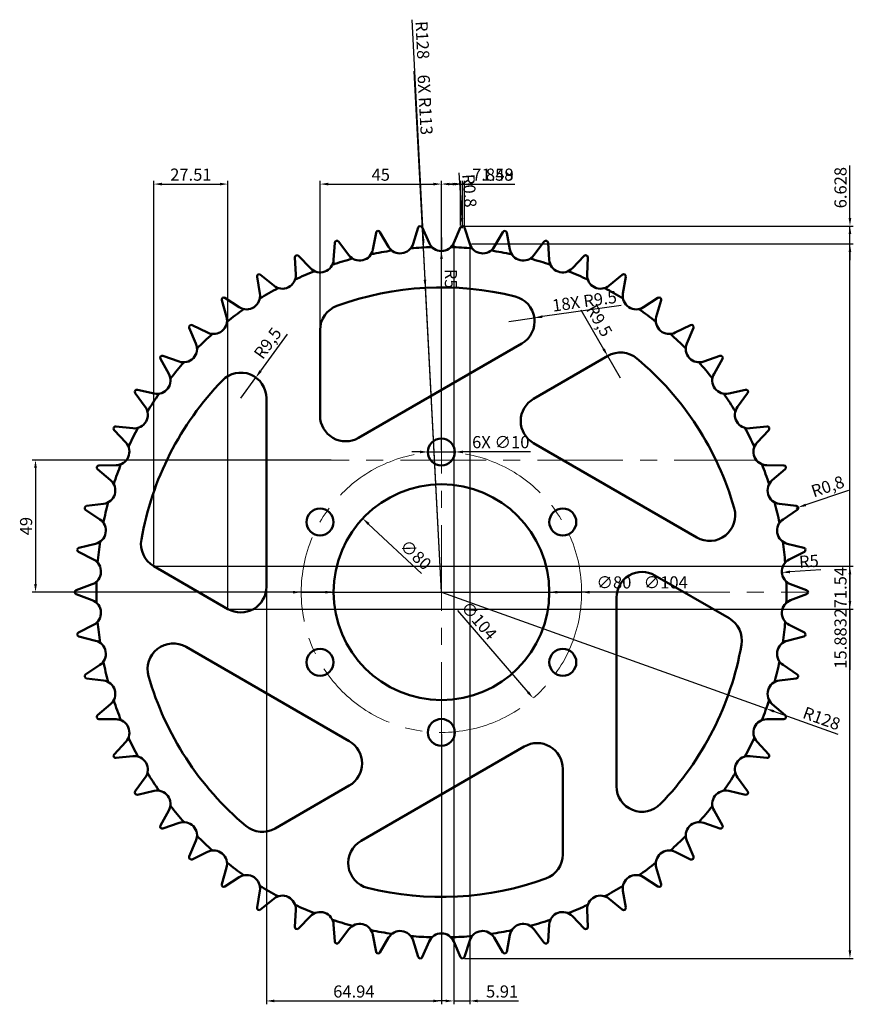
# Model space of a CAD drawing. Units: millimetres. Extents: x 3295 to 3604, y 1595 to 1960.
import ezdxf

# ---------------------------------------------------------------- set-up
doc = ezdxf.new("R2010")
doc.units = ezdxf.units.MM
doc.linetypes.add('CENTER', pattern=[50.8, 31.75, -6.35, 6.35, -6.35])
for name, color, linetype, lineweight in [('M-CNTR', 1, 'CENTER', 18), ('M-DIMS', 2, 'Continuous', 25), ('M-OUTL', 7, 'Continuous', 50)]:
    doc.layers.add(name, color=color, linetype=linetype, lineweight=lineweight)
doc.styles.get("Standard").update_dxf_attribs({"font": 'arial.ttf'})
doc.dimstyles.new('ISO-25', dxfattribs={"dimtxt": 4.5, "dimasz": 3, "dimexe": 1.25, "dimexo": 0.625, "dimtad": 1, "dimtxsty": 'Standard', "dimcen": 2.5, "dimadec": 0, "dimazin": 0, "dimtfac": 1, "dimtmove": 0, "dimatfit": 3, "dimfxl": 1, "dimarcsym": 0})

# ---------------------------------------------------------------- blocks, each defined once
blk = doc.blocks.new('*D1')
at = {"layer": 'Defpoints', "color": 0, "transparency": 16777216}
for p in [(3422.39, 1774.85), (3480.79, 1720.18)]:
    blk.add_point(p, dxfattribs=at)
at = {"layer": 'M-DIMS', "color": 0, "lineweight": -2, "transparency": 16777216}
blk.add_line((3444.18, 1754.46), (3424.58, 1772.8), dxfattribs=at)
at = {"layer": 'M-DIMS', "color": 0, "transparency": 16777216}
blk.add_solid([(3424.92, 1773.17), (3424.24, 1772.44), (3422.39, 1774.85)], dxfattribs=at)
at = {"layer": 'M-DIMS', "color": 0, "transparency": 16777216, "insert": (3441.67, 1760.98), "char_height": 4.5, "attachment_point": 5, "rotation": 316.8906}
blk.add_mtext('∅80', dxfattribs=at)
blk = doc.blocks.new('*D2')
at = {"layer": 'Defpoints', "color": 0, "transparency": 16777216}
for p in [(3417.54, 1786.82), (3485.64, 1708.22)]:
    blk.add_point(p, dxfattribs=at)
at = {"layer": 'M-DIMS', "color": 0, "lineweight": -2, "transparency": 16777216}
blk.add_line((3457.5, 1740.7), (3483.68, 1710.48), dxfattribs=at)
at = {"layer": 'M-DIMS', "color": 0, "transparency": 16777216}
blk.add_solid([(3484.06, 1710.81), (3483.3, 1710.16), (3485.64, 1708.22)], dxfattribs=at)
at = {"layer": 'M-DIMS', "color": 0, "transparency": 16777216, "insert": (3465.06, 1736.62), "char_height": 4.5, "attachment_point": 5, "rotation": 310.9048}
blk.add_mtext('∅104', dxfattribs=at)
blk = doc.blocks.new('*D3')
at = {"layer": 'Defpoints', "color": 0, "transparency": 16777216}
for p in [(3513.27, 1835.09), (3518.04, 1826.87)]:
    blk.add_point(p, dxfattribs=at)
at = {"layer": 'M-DIMS', "color": 0, "lineweight": -2, "transparency": 16777216}
for p, q in [((3503.33, 1852.19), (3511.76, 1837.68)), ((3518.04, 1826.87), (3513.27, 1835.09))]:
    blk.add_line(p, q, dxfattribs=at)
blk.add_arc((3518.04, 1826.87), 9.5, 120, 127.6887, dxfattribs=at)
at = {"layer": 'M-DIMS', "color": 0, "transparency": 16777216}
blk.add_solid([(3512.19, 1837.93), (3511.33, 1837.43), (3513.27, 1835.09)], dxfattribs=at)
at = {"layer": 'M-DIMS', "color": 0, "transparency": 16777216, "insert": (3509.67, 1847.91), "char_height": 4.5, "attachment_point": 5, "rotation": 300.1498}
blk.add_mtext('R9,5', dxfattribs=at)
blk = doc.blocks.new('*D4')
at = {"layer": 'Defpoints', "color": 0, "transparency": 16777216}
for p in [(3382.74, 1827.12), (3377.16, 1819.43)]:
    blk.add_point(p, dxfattribs=at)
at = {"layer": 'M-DIMS', "color": 0, "lineweight": -2, "transparency": 16777216}
for p, q in [((3394.37, 1843.13), (3384.5, 1829.55)), ((3377.16, 1819.43), (3382.74, 1827.12))]:
    blk.add_line(p, q, dxfattribs=at)
at = {"layer": 'M-DIMS', "color": 0, "transparency": 16777216}
blk.add_solid([(3384.1, 1829.84), (3384.91, 1829.25), (3382.74, 1827.12)], dxfattribs=at)
at = {"layer": 'M-DIMS', "color": 0, "transparency": 16777216, "insert": (3387.62, 1839.51), "char_height": 4.5, "attachment_point": 5, "rotation": 54.0064}
blk.add_mtext('R9,5', dxfattribs=at)
blk = doc.blocks.new('*D5')
at = {"layer": 'Defpoints', "color": 0, "transparency": 16777216}
for p in [(3583.15, 1778.69), (3583.91, 1778.95)]:
    blk.add_point(p, dxfattribs=at)
at = {"layer": 'M-DIMS', "color": 0, "lineweight": -2, "transparency": 16777216}
for p, q in [((3602.64, 1785.23), (3586.75, 1779.9)), ((3583.15, 1778.69), (3583.91, 1778.95))]:
    blk.add_line(p, q, dxfattribs=at)
at = {"layer": 'M-DIMS', "color": 0, "transparency": 16777216}
blk.add_solid([(3586.59, 1780.38), (3586.91, 1779.43), (3583.91, 1778.95)], dxfattribs=at)
at = {"layer": 'M-DIMS', "color": 0, "transparency": 16777216, "insert": (3595.06, 1786.2), "char_height": 4.5, "attachment_point": 5, "rotation": 18.5456}
blk.add_mtext('R0,8', dxfattribs=at)
blk = doc.blocks.new('*D6')
at = {"layer": 'Defpoints', "color": 0, "transparency": 16777216}
for p in [(3577.88, 1754.84), (3582.87, 1755.16)]:
    blk.add_point(p, dxfattribs=at)
at = {"layer": 'M-DIMS', "color": 0, "lineweight": -2, "transparency": 16777216}
blk.add_line((3592.39, 1755.78), (3580.87, 1755.03), dxfattribs=at)
at = {"layer": 'M-DIMS', "color": 0, "transparency": 16777216}
blk.add_solid([(3580.84, 1755.53), (3580.91, 1754.54), (3577.88, 1754.84)], dxfattribs=at)
at = {"layer": 'M-DIMS', "color": 0, "transparency": 16777216, "insert": (3587.94, 1758.41), "char_height": 4.5, "attachment_point": 5, "rotation": 3.7256}
blk.add_mtext('R5', dxfattribs=at)
blk = doc.blocks.new('*D7')
at = {"layer": 'Defpoints', "color": 0, "transparency": 16777216}
for p in [(3451.59, 1747.52), (3572.1, 1704.36)]:
    blk.add_point(p, dxfattribs=at)
at = {"layer": 'M-DIMS', "color": 0, "lineweight": -2, "transparency": 16777216}
for p, q in [((3451.59, 1747.52), (3572.1, 1704.36)), ((3598.76, 1694.8), (3574.92, 1703.34))]:
    blk.add_line(p, q, dxfattribs=at)
at = {"layer": 'M-DIMS', "color": 0, "transparency": 16777216}
blk.add_solid([(3575.09, 1703.82), (3574.75, 1702.87), (3572.1, 1704.36)], dxfattribs=at)
at = {"layer": 'M-DIMS', "color": 0, "transparency": 16777216, "insert": (3592.45, 1700.17), "char_height": 4.5, "attachment_point": 5, "rotation": 340.2933}
blk.add_mtext('R128', dxfattribs=at)
blk = doc.blocks.new('*D8')
at = {"layer": 'Defpoints', "color": 0, "transparency": 16777216}
for p in [(3411.27, 1796.52), (3301.02, 1747.52), (3411.27, 1747.52)]:
    blk.add_point(p, dxfattribs=at)
at = {"layer": 'M-DIMS', "color": 0, "lineweight": -2, "transparency": 16777216}
for p, q in [((3410.64, 1796.52), (3299.77, 1796.52)), ((3301.02, 1793.52), (3301.02, 1750.52)), ((3410.64, 1747.52), (3299.77, 1747.52))]:
    blk.add_line(p, q, dxfattribs=at)
at = {"layer": 'M-DIMS', "color": 0, "transparency": 16777216}
for points in [[(3300.52, 1793.52), (3301.52, 1793.52), (3301.02, 1796.52)], [(3300.52, 1750.52), (3301.52, 1750.52), (3301.02, 1747.52)]]:
    blk.add_solid(points, dxfattribs=at)
at = {"layer": 'M-DIMS', "color": 0, "transparency": 16777216, "insert": (3298.1, 1772.02), "char_height": 4.5, "attachment_point": 5, "rotation": 90}
blk.add_mtext('49', dxfattribs=at)
blk = doc.blocks.new('*D9')
at = {"layer": 'Defpoints', "color": 0, "transparency": 16777216}
for p in [(3459.5, 1883.29), (3603.14, 1883.29), (3459.5, 1611.75)]:
    blk.add_point(p, dxfattribs=at)
at = {"layer": 'M-DIMS', "color": 0, "lineweight": -2, "transparency": 16777216}
for p, q in [((3460.12, 1883.29), (3604.39, 1883.29)), ((3603.14, 1614.75), (3603.14, 1880.29)), ((3460.12, 1611.75), (3604.39, 1611.75))]:
    blk.add_line(p, q, dxfattribs=at)
at = {"layer": 'M-DIMS', "color": 0, "transparency": 16777216}
for points in [[(3602.64, 1880.29), (3603.64, 1880.29), (3603.14, 1883.29)], [(3602.64, 1614.75), (3603.64, 1614.75), (3603.14, 1611.75)]]:
    blk.add_solid(points, dxfattribs=at)
at = {"layer": 'M-DIMS', "color": 0, "transparency": 16777216, "insert": (3600.22, 1747.52), "char_height": 4.5, "attachment_point": 5, "rotation": 90}
blk.add_mtext('271.54', dxfattribs=at)
blk = doc.blocks.new('*D10')
at = {"layer": 'Defpoints', "color": 0, "transparency": 16777216}
for p in [(3386.66, 1749.5), (3451.59, 1695.52), (3451.59, 1595.97)]:
    blk.add_point(p, dxfattribs=at)
at = {"layer": 'M-DIMS', "color": 0, "lineweight": -2, "transparency": 16777216}
for p, q in [((3386.66, 1748.88), (3386.66, 1594.72)), ((3451.59, 1694.89), (3451.59, 1594.72)), ((3389.66, 1595.97), (3448.59, 1595.97))]:
    blk.add_line(p, q, dxfattribs=at)
at = {"layer": 'M-DIMS', "color": 0, "transparency": 16777216}
for points in [[(3389.66, 1596.47), (3389.66, 1595.47), (3386.66, 1595.97)], [(3448.59, 1596.47), (3448.59, 1595.47), (3451.59, 1595.97)]]:
    blk.add_solid(points, dxfattribs=at)
at = {"layer": 'M-DIMS', "color": 0, "transparency": 16777216, "insert": (3419.12, 1598.89), "char_height": 4.5, "attachment_point": 5}
blk.add_mtext('64.94', dxfattribs=at)
blk = doc.blocks.new('*D11')
at = {"layer": 'Defpoints', "color": 0, "transparency": 16777216}
for p in [(3451.59, 1898.84), (3406.59, 1844.74), (3451.59, 1799.52)]:
    blk.add_point(p, dxfattribs=at)
at = {"layer": 'M-DIMS', "color": 0, "lineweight": -2, "transparency": 16777216}
for p, q in [((3406.59, 1845.36), (3406.59, 1900.09)), ((3409.59, 1898.84), (3448.59, 1898.84)), ((3451.59, 1800.14), (3451.59, 1900.09))]:
    blk.add_line(p, q, dxfattribs=at)
at = {"layer": 'M-DIMS', "color": 0, "transparency": 16777216}
for points in [[(3409.59, 1899.34), (3409.59, 1898.34), (3406.59, 1898.84)], [(3448.59, 1899.34), (3448.59, 1898.34), (3451.59, 1898.84)]]:
    blk.add_solid(points, dxfattribs=at)
at = {"layer": 'M-DIMS', "color": 0, "transparency": 16777216, "insert": (3429.09, 1901.75), "char_height": 4.5, "attachment_point": 5}
blk.add_mtext('45', dxfattribs=at)
blk = doc.blocks.new('*D12')
at = {"layer": 'Defpoints', "color": 0, "transparency": 16777216}
for p in [(3372.41, 1898.84), (3344.9, 1757.16), (3372.41, 1741.27)]:
    blk.add_point(p, dxfattribs=at)
at = {"layer": 'M-DIMS', "color": 0, "lineweight": -2, "transparency": 16777216}
for p, q in [((3344.9, 1757.78), (3344.9, 1900.09)), ((3347.9, 1898.84), (3369.41, 1898.84)), ((3372.41, 1741.9), (3372.41, 1900.09))]:
    blk.add_line(p, q, dxfattribs=at)
at = {"layer": 'M-DIMS', "color": 0, "transparency": 16777216}
for points in [[(3347.9, 1899.34), (3347.9, 1898.34), (3344.9, 1898.84)], [(3369.41, 1899.34), (3369.41, 1898.34), (3372.41, 1898.84)]]:
    blk.add_solid(points, dxfattribs=at)
at = {"layer": 'M-DIMS', "color": 0, "transparency": 16777216, "insert": (3358.65, 1901.76), "char_height": 4.5, "attachment_point": 5}
blk.add_mtext('27.51', dxfattribs=at)
blk = doc.blocks.new('*D13')
at = {"layer": 'Defpoints', "color": 0, "transparency": 16777216}
for p in [(3344.9, 1757.16), (3372.41, 1741.27), (3603.14, 1741.27)]:
    blk.add_point(p, dxfattribs=at)
at = {"layer": 'M-DIMS', "color": 0, "lineweight": -2, "transparency": 16777216}
for p, q in [((3345.52, 1757.16), (3604.39, 1757.16)), ((3603.14, 1754.16), (3603.14, 1744.27)), ((3373.03, 1741.27), (3604.39, 1741.27)), ((3603.14, 1741.27), (3603.14, 1718.77))]:
    blk.add_line(p, q, dxfattribs=at)
at = {"layer": 'M-DIMS', "color": 0, "transparency": 16777216}
for points in [[(3602.64, 1754.16), (3603.64, 1754.16), (3603.14, 1757.16)], [(3602.64, 1744.27), (3603.64, 1744.27), (3603.14, 1741.27)]]:
    blk.add_solid(points, dxfattribs=at)
at = {"layer": 'M-DIMS', "color": 0, "transparency": 16777216, "insert": (3600.22, 1728.52), "char_height": 4.5, "attachment_point": 5, "rotation": 90}
blk.add_mtext('15.883', dxfattribs=at)
blk = doc.blocks.new('*D14')
at = {"layer": 'Defpoints', "color": 0, "transparency": 16777216}
for p in [(3459.45, 1898.84), (3459.45, 1882.49), (3451.59, 1879.02)]:
    blk.add_point(p, dxfattribs=at)
at = {"layer": 'M-DIMS', "color": 0, "lineweight": -2, "transparency": 16777216}
for p, q in [((3451.59, 1879.64), (3451.59, 1900.09)), ((3454.59, 1898.84), (3456.45, 1898.84)), ((3459.45, 1883.11), (3459.45, 1900.09)), ((3459.45, 1898.84), (3478.86, 1898.84))]:
    blk.add_line(p, q, dxfattribs=at)
at = {"layer": 'M-DIMS', "color": 0, "transparency": 16777216}
for points in [[(3454.59, 1899.34), (3454.59, 1898.34), (3451.59, 1898.84)], [(3456.45, 1899.34), (3456.45, 1898.34), (3459.45, 1898.84)]]:
    blk.add_solid(points, dxfattribs=at)
at = {"layer": 'M-DIMS', "color": 0, "transparency": 16777216, "insert": (3470.65, 1901.76), "char_height": 4.5, "attachment_point": 5}
blk.add_mtext('7.858', dxfattribs=at)
blk = doc.blocks.new('*D15')
at = {"layer": 'Defpoints', "color": 0, "transparency": 16777216}
for p in [(3456.17, 1877), (3462.08, 1876.66), (3462.08, 1595.97)]:
    blk.add_point(p, dxfattribs=at)
at = {"layer": 'M-DIMS', "color": 0, "lineweight": -2, "transparency": 16777216}
for p, q in [((3456.17, 1876.38), (3456.17, 1594.72)), ((3462.08, 1876.04), (3462.08, 1594.72)), ((3453.17, 1595.97), (3450.17, 1595.97)), ((3456.17, 1595.97), (3462.08, 1595.97)), ((3465.08, 1595.97), (3480.15, 1595.97))]:
    blk.add_line(p, q, dxfattribs=at)
at = {"layer": 'M-DIMS', "color": 0, "transparency": 16777216}
for points in [[(3453.17, 1596.47), (3453.17, 1595.47), (3456.17, 1595.97)], [(3465.08, 1596.47), (3465.08, 1595.47), (3462.08, 1595.97)]]:
    blk.add_solid(points, dxfattribs=at)
at = {"layer": 'M-DIMS', "color": 0, "transparency": 16777216, "insert": (3474.11, 1598.89), "char_height": 4.5, "attachment_point": 5}
blk.add_mtext('5.91', dxfattribs=at)
blk = doc.blocks.new('*D16')
at = {"layer": 'Defpoints', "color": 0, "transparency": 16777216}
for p in [(3460.21, 1898.84), (3458.72, 1882.81), (3460.21, 1882.72)]:
    blk.add_point(p, dxfattribs=at)
at = {"layer": 'M-DIMS', "color": 0, "lineweight": -2, "transparency": 16777216}
for p, q in [((3455.72, 1898.84), (3452.72, 1898.84)), ((3458.72, 1883.44), (3458.72, 1900.09)), ((3458.72, 1898.84), (3460.21, 1898.84)), ((3460.21, 1883.35), (3460.21, 1900.09)), ((3463.21, 1898.84), (3478.74, 1898.84))]:
    blk.add_line(p, q, dxfattribs=at)
at = {"layer": 'M-DIMS', "color": 0, "transparency": 16777216}
for points in [[(3455.72, 1899.34), (3455.72, 1898.34), (3458.72, 1898.84)], [(3463.21, 1899.34), (3463.21, 1898.34), (3460.21, 1898.84)]]:
    blk.add_solid(points, dxfattribs=at)
at = {"layer": 'M-DIMS', "color": 0, "transparency": 16777216, "insert": (3472.48, 1901.76), "char_height": 4.5, "attachment_point": 5}
blk.add_mtext('1.49', dxfattribs=at)
blk = doc.blocks.new('*D17')
at = {"layer": 'Defpoints', "color": 0, "transparency": 16777216}
for p in [(3459.5, 1883.29), (3603.14, 1883.29), (3462.08, 1876.66)]:
    blk.add_point(p, dxfattribs=at)
at = {"layer": 'M-DIMS', "color": 0, "lineweight": -2, "transparency": 16777216}
for p, q in [((3603.14, 1886.29), (3603.14, 1905.76)), ((3460.12, 1883.29), (3604.39, 1883.29)), ((3603.14, 1876.66), (3603.14, 1883.29)), ((3462.7, 1876.66), (3604.39, 1876.66)), ((3603.14, 1873.66), (3603.14, 1870.66))]:
    blk.add_line(p, q, dxfattribs=at)
at = {"layer": 'M-DIMS', "color": 0, "transparency": 16777216}
for points in [[(3602.64, 1886.29), (3603.64, 1886.29), (3603.14, 1883.29)], [(3602.64, 1873.66), (3603.64, 1873.66), (3603.14, 1876.66)]]:
    blk.add_solid(points, dxfattribs=at)
at = {"layer": 'M-DIMS', "color": 0, "transparency": 16777216, "insert": (3600.22, 1897.52), "char_height": 4.5, "attachment_point": 5, "rotation": 90}
blk.add_mtext('6.628', dxfattribs=at)
blk = doc.blocks.new('*D18')
at = {"layer": 'Defpoints', "color": 0, "transparency": 16777216}
for p in [(3445.63, 1860.36), (3451.59, 1747.52)]:
    blk.add_point(p, dxfattribs=at)
at = {"layer": 'M-DIMS', "color": 0, "lineweight": -2, "transparency": 16777216}
for p, q in [((3441.39, 1940.65), (3445.47, 1863.36)), ((3451.59, 1747.52), (3445.63, 1860.36))]:
    blk.add_line(p, q, dxfattribs=at)
at = {"layer": 'M-DIMS', "color": 0, "transparency": 16777216}
blk.add_solid([(3445.97, 1863.38), (3444.97, 1863.33), (3445.63, 1860.36)], dxfattribs=at)
at = {"layer": 'M-DIMS', "color": 0, "transparency": 16777216, "insert": (3444.98, 1928.22), "char_height": 4.5, "attachment_point": 5, "rotation": 273.0233}
blk.add_mtext('6X R113', dxfattribs=at)
blk = doc.blocks.new('*D19')
at = {"layer": 'Defpoints', "color": 0, "transparency": 16777216}
for p in [(3399.59, 1747.52), (3503.59, 1747.52)]:
    blk.add_point(p, dxfattribs=at)
at = {"layer": 'M-DIMS', "color": 0, "lineweight": -2, "transparency": 16777216}
for p, q in [((3396.59, 1747.52), (3393.59, 1747.52)), ((3399.59, 1747.52), (3503.59, 1747.52)), ((3542.83, 1747.52), (3506.59, 1747.52))]:
    blk.add_line(p, q, dxfattribs=at)
at = {"layer": 'M-DIMS', "color": 0, "transparency": 16777216}
for points in [[(3396.59, 1748.02), (3396.59, 1747.02), (3399.59, 1747.52)], [(3506.59, 1748.02), (3506.59, 1747.02), (3503.59, 1747.52)]]:
    blk.add_solid(points, dxfattribs=at)
at = {"layer": 'M-DIMS', "color": 0, "transparency": 16777216, "insert": (3534.79, 1750.57), "char_height": 4.5, "attachment_point": 5, "rotation": 359.9995}
blk.add_mtext('∅104', dxfattribs=at)
blk = doc.blocks.new('*D20')
at = {"layer": 'Defpoints', "color": 0, "transparency": 16777216}
for p in [(3411.59, 1747.52), (3491.59, 1747.52)]:
    blk.add_point(p, dxfattribs=at)
at = {"layer": 'M-DIMS', "color": 0, "lineweight": -2, "transparency": 16777216}
for p, q in [((3408.59, 1747.52), (3405.59, 1747.52)), ((3411.59, 1747.52), (3491.59, 1747.52)), ((3521.88, 1747.52), (3494.59, 1747.52))]:
    blk.add_line(p, q, dxfattribs=at)
at = {"layer": 'M-DIMS', "color": 0, "transparency": 16777216}
for points in [[(3408.59, 1748.02), (3408.59, 1747.02), (3411.59, 1747.52)], [(3494.59, 1748.02), (3494.59, 1747.02), (3491.59, 1747.52)]]:
    blk.add_solid(points, dxfattribs=at)
at = {"layer": 'M-DIMS', "color": 0, "transparency": 16777216, "insert": (3515.59, 1750.57), "char_height": 4.5, "attachment_point": 5, "rotation": 359.9994}
blk.add_mtext('∅80', dxfattribs=at)
blk = doc.blocks.new('*D21')
at = {"layer": 'Defpoints', "color": 0, "transparency": 16777216}
for p in [(3476.65, 1847.94), (3486.06, 1849.26)]:
    blk.add_point(p, dxfattribs=at)
at = {"layer": 'M-DIMS', "color": 0, "lineweight": -2, "transparency": 16777216}
for p, q in [((3518.27, 1853.78), (3489.03, 1849.68)), ((3476.65, 1847.94), (3486.06, 1849.26))]:
    blk.add_line(p, q, dxfattribs=at)
at = {"layer": 'M-DIMS', "color": 0, "transparency": 16777216}
blk.add_solid([(3488.96, 1850.17), (3489.1, 1849.18), (3486.06, 1849.26)], dxfattribs=at)
at = {"layer": 'M-DIMS', "color": 0, "transparency": 16777216, "insert": (3504.73, 1854.83), "char_height": 4.5, "attachment_point": 5, "rotation": 7.9916}
blk.add_mtext('18X R9.5', dxfattribs=at)
blk = doc.blocks.new('*D22')
at = {"layer": 'Defpoints', "color": 0, "transparency": 16777216}
for p in [(3446.59, 1799.52), (3456.59, 1799.52)]:
    blk.add_point(p, dxfattribs=at)
at = {"layer": 'M-DIMS', "color": 0, "lineweight": -2, "transparency": 16777216}
for p, q in [((3443.59, 1799.52), (3440.59, 1799.52)), ((3446.59, 1799.52), (3456.59, 1799.52)), ((3484.62, 1799.52), (3459.59, 1799.52))]:
    blk.add_line(p, q, dxfattribs=at)
at = {"layer": 'M-DIMS', "color": 0, "transparency": 16777216}
for points in [[(3443.59, 1800.02), (3443.59, 1799.02), (3446.59, 1799.52)], [(3459.59, 1800.02), (3459.59, 1799.02), (3456.59, 1799.52)]]:
    blk.add_solid(points, dxfattribs=at)
at = {"layer": 'M-DIMS', "color": 0, "transparency": 16777216, "insert": (3473.61, 1802.57), "char_height": 4.5, "attachment_point": 5, "rotation": 359.9952}
blk.add_mtext('6X ∅10', dxfattribs=at)
blk = doc.blocks.new('*D23')
at = {"layer": 'Defpoints', "color": 0, "transparency": 16777216}
for p in [(3459.4, 1883.29), (3459.46, 1882.49)]:
    blk.add_point(p, dxfattribs=at)
at = {"layer": 'M-DIMS', "color": 0, "lineweight": -2, "transparency": 16777216}
for p, q in [((3458.04, 1903), (3459.19, 1886.28)), ((3459.46, 1882.49), (3459.4, 1883.29))]:
    blk.add_line(p, q, dxfattribs=at)
at = {"layer": 'M-DIMS', "color": 0, "transparency": 16777216}
blk.add_solid([(3459.69, 1886.31), (3458.7, 1886.25), (3459.4, 1883.29)], dxfattribs=at)
at = {"layer": 'M-DIMS', "color": 0, "transparency": 16777216, "insert": (3461.43, 1896.34), "char_height": 4.5, "attachment_point": 5, "rotation": 273.9409}
blk.add_mtext('R0.8', dxfattribs=at)
blk = doc.blocks.new('*D24')
at = {"layer": 'Defpoints', "color": 0, "transparency": 16777216}
for p in [(3451.59, 1879.02), (3451.6, 1874.02)]:
    blk.add_point(p, dxfattribs=at)
at = {"layer": 'M-DIMS', "color": 0, "lineweight": -2, "transparency": 16777216}
for p, q in [((3451.59, 1879.02), (3451.6, 1874.02)), ((3451.62, 1859.48), (3451.6, 1871.02))]:
    blk.add_line(p, q, dxfattribs=at)
at = {"layer": 'M-DIMS', "color": 0, "transparency": 16777216}
blk.add_solid([(3452.1, 1871.02), (3451.1, 1871.02), (3451.6, 1874.02)], dxfattribs=at)
at = {"layer": 'M-DIMS', "color": 0, "transparency": 16777216, "insert": (3454.53, 1863.75), "char_height": 4.5, "attachment_point": 5, "rotation": 270.0928}
blk.add_mtext('R5', dxfattribs=at)
blk = doc.blocks.new('*D25')
at = {"layer": 'Defpoints', "color": 0, "transparency": 16777216}
for p in [(3445, 1875.35), (3451.59, 1747.52)]:
    blk.add_point(p, dxfattribs=at)
at = {"layer": 'M-DIMS', "color": 0, "lineweight": -2, "transparency": 16777216}
for p, q in [((3440.65, 1959.79), (3444.85, 1878.34)), ((3451.59, 1747.52), (3445, 1875.35))]:
    blk.add_line(p, q, dxfattribs=at)
at = {"layer": 'M-DIMS', "color": 0, "transparency": 16777216}
blk.add_solid([(3445.35, 1878.37), (3444.35, 1878.32), (3445, 1875.35)], dxfattribs=at)
at = {"layer": 'M-DIMS', "color": 0, "transparency": 16777216, "insert": (3443.97, 1952.2), "char_height": 4.5, "attachment_point": 5, "rotation": 272.9515}
blk.add_mtext('R128', dxfattribs=at)

msp = doc.modelspace()

# ---------------------------------------------------------------- linework, layer by layer
at = {"layer": 'M-CNTR'}
for p, q in [((3451.5919, 1874.0184), (3451.5919, 1611.5184)), ((3334.7817, 1796.5184), (3568.4021, 1796.5184)), ((3323.5919, 1747.5184), (3587.5919, 1747.5184))]:
    msp.add_line(p, q, dxfattribs=at)
msp.add_circle((3451.5919, 1747.5184), 52, dxfattribs=at)
at = {"layer": 'M-OUTL'}
for points in [[(3412.5839, 1877.8042, -0.3133068), (3413.4516, 1877.5202), (3417.2771, 1872.4589, 0.65251373), (3426.1835, 1874.5698), (3427.3306, 1880.8096, -0.3133068), (3427.9785, 1881.4528)], [(3427.973, 1881.4518, -0.3133068), (3428.8018, 1881.069), (3432.0138, 1875.5978, 0.65251373), (3441.105, 1876.6605), (3442.9688, 1882.7249, -0.3133068), (3443.687, 1883.2885)], [(3443.6814, 1883.2882, -0.3133068), (3444.4602, 1882.8117), (3447.0153, 1877.0047, 0.65251373), (3456.1684, 1877.0047), (3458.7236, 1882.8117, -0.3133068), (3459.5024, 1883.2882)], [(3459.4968, 1883.2885, -0.3133068), (3460.215, 1882.7249), (3462.0787, 1876.6605, 0.65251373), (3471.1699, 1875.5978), (3474.382, 1881.069, -0.3133068), (3475.2108, 1881.4518)], [(3475.2053, 1881.4528, -0.3133068), (3475.8532, 1880.8096), (3477.0003, 1874.5698, 0.65251373), (3485.9067, 1872.4589), (3489.7321, 1877.5202, -0.3133068), (3490.5998, 1877.8042)], [(3397.7225, 1872.3947, -0.3133068), (3398.6172, 1872.2133), (3403.0044, 1867.6304, 0.65251373), (3411.6055, 1870.761), (3412.0205, 1877.0917, -0.3133068), (3412.5893, 1877.8058)], [(3490.5944, 1877.8058, -0.3133068), (3491.1633, 1877.0917), (3491.5782, 1870.761, 0.65251373), (3500.1793, 1867.6304), (3504.5665, 1872.2133, -0.3133068), (3505.4613, 1872.3947)], [(3383.5894, 1865.2965, -0.3133068), (3384.4992, 1865.2202), (3389.3888, 1861.1776, 0.65251373), (3397.5683, 1865.2855), (3397.2455, 1871.6216, -0.3133068), (3397.7276, 1872.3969)], [(3505.4561, 1872.3969, -0.3133068), (3505.9383, 1871.6216), (3505.6154, 1865.2855, 0.65251373), (3513.795, 1861.1776), (3518.6845, 1865.2202, -0.3133068), (3519.5943, 1865.2965)], [(3370.3761, 1856.6055, -0.3133068), (3371.2885, 1856.6354), (3376.6143, 1853.1878, 0.65251373), (3384.2617, 1858.2175), (3383.2054, 1864.4733, -0.3133068), (3383.5943, 1865.2993)], [(3519.5894, 1865.2993, -0.3133068), (3519.9783, 1864.4733), (3518.9221, 1858.2175, 0.65251373), (3526.5694, 1853.1878), (3531.8952, 1856.6354, -0.3133068), (3532.8077, 1856.6055)], [(3358.261, 1846.4393, -0.3133068), (3359.1638, 1846.5749), (3364.8539, 1843.7689, 0.65251373), (3371.8656, 1849.6524), (3370.0902, 1855.7433, -0.3133068), (3370.3806, 1856.6088)], [(3532.8032, 1856.6088, -0.3133068), (3533.0935, 1855.7433), (3531.3182, 1849.6524, 0.65251373), (3538.3299, 1843.7689), (3544.0199, 1846.5749, -0.3133068), (3544.9228, 1846.4393)], [(3347.408, 1834.9354, -0.3133068), (3348.289, 1835.1749), (3354.2664, 1833.0484, 0.65251373), (3360.5476, 1839.7062), (3358.0772, 1845.5497, -0.3133068), (3358.265, 1846.4432)], [(3544.9187, 1846.4432, -0.3133068), (3545.1066, 1845.5497), (3542.6361, 1839.7062, 0.65251373), (3548.9174, 1833.0484), (3554.8947, 1835.1749, -0.3133068), (3555.7757, 1834.9354)], [(3337.964, 1822.2493, -0.3133068), (3338.8112, 1822.5895), (3344.995, 1821.1713, 0.65251373), (3350.4609, 1828.5132), (3347.3287, 1834.0305, -0.3133068), (3347.4116, 1834.9397)], [(3555.7721, 1834.9397, -0.3133068), (3555.855, 1834.0305), (3552.7229, 1828.5132, 0.65251373), (3558.1887, 1821.1713), (3564.3725, 1822.5895, -0.3133068), (3565.2198, 1822.2493)], [(3330.0566, 1808.5526, -0.3133068), (3330.8586, 1808.9888), (3337.1652, 1808.2981, 0.65251373), (3341.7418, 1816.225), (3337.9903, 1821.3413, -0.3133068), (3337.9671, 1822.254)], [(3565.2167, 1822.254, -0.3133068), (3565.1934, 1821.3413), (3561.442, 1816.225, 0.65251373), (3566.0185, 1808.2981), (3572.3252, 1808.9888, -0.3133068), (3573.1272, 1808.5526)], [(3323.7927, 1794.0305, -0.3133068), (3324.5387, 1794.5569), (3330.8828, 1794.603, 0.65251373), (3334.5082, 1803.0076), (3330.1881, 1807.6538, -0.3133068), (3330.0591, 1808.5576)], [(3573.1247, 1808.5576, -0.3133068), (3572.9956, 1807.6538), (3568.6756, 1803.0076, 0.65251373), (3572.3009, 1794.603), (3578.6451, 1794.5569, -0.3133068), (3579.391, 1794.0305)], [(3319.2571, 1778.8794, -0.3133068), (3319.9369, 1779.4889), (3326.2328, 1780.2712, 0.65251373), (3328.858, 1789.0398), (3324.0277, 1793.1531, -0.3133068), (3323.7946, 1794.0358)], [(3579.3891, 1794.0358, -0.3133068), (3579.156, 1793.1531), (3574.3258, 1789.0398, 0.65251373), (3576.9509, 1780.2712), (3583.2468, 1779.4889, -0.3133068), (3583.9266, 1778.8794)], [(3316.5111, 1763.3043, -0.3133068), (3317.1156, 1763.9885), (3323.2781, 1765.4964, 0.65251373), (3324.8675, 1774.5105), (3319.5924, 1778.0352, -0.3133068), (3319.2584, 1778.8849)], [(3583.9253, 1778.8849, -0.3133068), (3583.5914, 1778.0352), (3578.3162, 1774.5105, 0.65251373), (3579.9057, 1765.4964), (3586.0682, 1763.9885, -0.3133068), (3586.6726, 1763.3043)], [(3315.5919, 1747.5156, -0.3133068), (3316.1128, 1748.2654), (3322.0586, 1750.4786, 0.65251373), (3322.5908, 1759.6162), (3316.9421, 1762.5047, -0.3133068), (3316.5118, 1763.3098)], [(3586.672, 1763.3098, -0.3133068), (3586.2416, 1762.5047), (3580.593, 1759.6162, 0.65251373), (3581.1252, 1750.4786), (3587.0709, 1748.2654, -0.3133068), (3587.5919, 1747.5156)], [(3316.5118, 1731.727, -0.3133068), (3316.9421, 1732.5322), (3322.5908, 1735.4206, 0.65251373), (3322.0586, 1744.5583), (3316.1128, 1746.7715, -0.3133068), (3315.5919, 1747.5212)], [(3587.5919, 1747.5212, -0.3133068), (3587.0709, 1746.7715), (3581.1252, 1744.5583, 0.65251373), (3580.593, 1735.4206), (3586.2416, 1732.5322, -0.3133068), (3586.672, 1731.727)], [(3319.2584, 1716.1519, -0.3133068), (3319.5924, 1717.0016), (3324.8675, 1720.5263, 0.65251373), (3323.2781, 1729.5404), (3317.1156, 1731.0483, -0.3133068), (3316.5111, 1731.7326)], [(3586.6726, 1731.7326, -0.3133068), (3586.0682, 1731.0483), (3579.9057, 1729.5404, 0.65251373), (3578.3162, 1720.5263), (3583.5914, 1717.0016, -0.3133068), (3583.9253, 1716.1519)], [(3323.7946, 1701.001, -0.3133068), (3324.0277, 1701.8838), (3328.858, 1705.997, 0.65251373), (3326.2328, 1714.7656), (3319.9369, 1715.548, -0.3133068), (3319.2571, 1716.1574)], [(3583.9266, 1716.1574, -0.3133068), (3583.2468, 1715.548), (3576.9509, 1714.7656, 0.65251373), (3574.3258, 1705.997), (3579.156, 1701.8838, -0.3133068), (3579.3891, 1701.001)], [(3330.0591, 1686.4792, -0.3133068), (3330.1881, 1687.383), (3334.5082, 1692.0293, 0.65251373), (3330.8828, 1700.4338), (3324.5387, 1700.4799, -0.3133068), (3323.7927, 1701.0063)], [(3579.391, 1701.0063, -0.3133068), (3578.6451, 1700.4799), (3572.3009, 1700.4338, 0.65251373), (3568.6756, 1692.0293), (3572.9956, 1687.383, -0.3133068), (3573.1247, 1686.4792)], [(3337.9671, 1672.7829, -0.3133068), (3337.9903, 1673.6955), (3341.7418, 1678.8119, 0.65251373), (3337.1652, 1686.7387), (3330.8586, 1686.048, -0.3133068), (3330.0566, 1686.4842)], [(3573.1272, 1686.4842, -0.3133068), (3572.3252, 1686.048), (3566.0185, 1686.7387, 0.65251373), (3561.442, 1678.8119), (3565.1934, 1673.6955, -0.3133068), (3565.2167, 1672.7829)], [(3347.4116, 1660.0972, -0.3133068), (3347.3287, 1661.0064), (3350.4609, 1666.5236, 0.65251373), (3344.995, 1673.8655), (3338.8112, 1672.4474, -0.3133068), (3337.964, 1672.7875)], [(3565.2198, 1672.7875, -0.3133068), (3564.3725, 1672.4474), (3558.1887, 1673.8655, 0.65251373), (3552.7229, 1666.5236), (3555.855, 1661.0064, -0.3133068), (3555.7721, 1660.0972)], [(3358.265, 1648.5937, -0.3133068), (3358.0772, 1649.4871), (3360.5476, 1655.3307, 0.65251373), (3354.2664, 1661.9884), (3348.289, 1659.8619, -0.3133068), (3347.408, 1660.1014)], [(3555.7757, 1660.1014, -0.3133068), (3554.8947, 1659.8619), (3548.9174, 1661.9884, 0.65251373), (3542.6361, 1655.3307), (3545.1066, 1649.4871, -0.3133068), (3544.9187, 1648.5937)], [(3370.3806, 1638.428, -0.3133068), (3370.0902, 1639.2936), (3371.8656, 1645.3844, 0.65251373), (3364.8539, 1651.2679), (3359.1638, 1648.4619, -0.3133068), (3358.261, 1648.5975)], [(3544.9228, 1648.5975, -0.3133068), (3544.0199, 1648.4619), (3538.3299, 1651.2679, 0.65251373), (3531.3182, 1645.3844), (3533.0935, 1639.2936, -0.3133068), (3532.8032, 1638.428)], [(3383.5943, 1629.7376, -0.3133068), (3383.2054, 1630.5636), (3384.2617, 1636.8194, 0.65251373), (3376.6143, 1641.8491), (3371.2885, 1638.4015, -0.3133068), (3370.3761, 1638.4313)], [(3532.8077, 1638.4313, -0.3133068), (3531.8952, 1638.4015), (3526.5694, 1641.8491, 0.65251373), (3518.9221, 1636.8194), (3519.9783, 1630.5636, -0.3133068), (3519.5894, 1629.7376)], [(3397.7276, 1622.6399, -0.3133068), (3397.2455, 1623.4152), (3397.5683, 1629.7513, 0.65251373), (3389.3888, 1633.8592), (3384.4992, 1629.8166, -0.3133068), (3383.5894, 1629.7404)], [(3519.5943, 1629.7404, -0.3133068), (3518.6845, 1629.8166), (3513.795, 1633.8592, 0.65251373), (3505.6154, 1629.7513), (3505.9383, 1623.4152, -0.3133068), (3505.4561, 1622.6399)], [(3412.5893, 1617.231, -0.3133068), (3412.0205, 1617.9451), (3411.6055, 1624.2759, 0.65251373), (3403.0044, 1627.4064), (3398.6172, 1622.8235, -0.3133068), (3397.7225, 1622.6421)], [(3505.4613, 1622.6421, -0.3133068), (3504.5665, 1622.8235), (3500.1793, 1627.4064, 0.65251373), (3491.5782, 1624.2759), (3491.1633, 1617.9451, -0.3133068), (3490.5944, 1617.231)], [(3427.9785, 1613.5841, -0.3133068), (3427.3306, 1614.2273), (3426.1835, 1620.467, 0.65251373), (3417.2771, 1622.5779), (3413.4516, 1617.5167, -0.3133068), (3412.5839, 1617.2326)], [(3443.687, 1611.7483, -0.3133068), (3442.9688, 1612.312), (3441.105, 1618.3764, 0.65251373), (3432.0138, 1619.439), (3428.8018, 1613.9679, -0.3133068), (3427.973, 1613.5851)], [(3459.5024, 1611.7487, -0.3133068), (3458.7236, 1612.2251), (3456.1684, 1618.0322, 0.65251373), (3447.0153, 1618.0322), (3444.4602, 1612.2251, -0.3133068), (3443.6814, 1611.7487)], [(3475.2108, 1613.5851, -0.3133068), (3474.382, 1613.9679), (3471.1699, 1619.439, 0.65251373), (3462.0787, 1618.3764), (3460.215, 1612.312, -0.3133068), (3459.4968, 1611.7483)], [(3490.5998, 1617.2326, -0.3133068), (3489.7321, 1617.5167), (3485.9067, 1622.5779, 0.65251373), (3477.0003, 1620.467), (3475.8532, 1614.2273, -0.3133068), (3475.2053, 1613.5841)]]:
    msp.add_lwpolyline(points, format="xyb", dxfattribs=at)
for points in [[(3481.4037, 1839.7111, 0.67442544), (3478.9541, 1857.1556, 0.14977464), (3412.8334, 1853.6635, 0.31501357), (3406.5919, 1844.7398), (3406.5919, 1812.9729, 0.57735027), (3420.8419, 1804.7457)], [(3546.339, 1767.7969, 0.67442544), (3560.2216, 1778.6406, 0.14977464), (3524.137, 1834.1568, 0.31501357), (3513.2881, 1835.1003), (3485.7771, 1819.2168, 0.57735027), (3485.7771, 1802.7623)], [(3386.6566, 1819.4326, 0.67442544), (3370.3244, 1826.0334, 0.14977464), (3340.2883, 1767.0252, 0.31501357), (3344.8957, 1757.158), (3372.4066, 1741.2745, 0.57735027), (3386.6566, 1749.5018)], [(3516.5271, 1675.6043, 0.67442544), (3532.8593, 1669.0035, 0.14977464), (3562.8955, 1728.0117, 0.31501357), (3558.2881, 1737.8789), (3530.7771, 1753.7623, 0.57735027), (3516.5271, 1745.5351)], [(3356.8448, 1727.2399, 0.67442544), (3342.9622, 1716.3962, 0.14977464), (3379.0467, 1660.8801, 0.31501357), (3389.8957, 1659.9366), (3417.4066, 1675.82, 0.57735027), (3417.4066, 1692.2745)], [(3421.78, 1655.3258, 0.67442544), (3424.2297, 1637.8812, 0.14977464), (3490.3503, 1641.3733, 0.31501357), (3496.5919, 1650.297), (3496.5919, 1682.0639, 0.57735027), (3482.3419, 1690.2912)]]:
    msp.add_lwpolyline(points, format="xyb", close=True, dxfattribs=at)
for centre, radius in [((3451.5919, 1799.5184), 5), ((3451.5919, 1747.5184), 40), ((3406.5586, 1773.5184), 5), ((3496.6252, 1773.5184), 5), ((3406.5586, 1721.5184), 5), ((3496.6252, 1721.5184), 5), ((3451.5919, 1695.5184), 5)]:
    msp.add_circle(centre, radius, dxfattribs=at)
for radius, start, end in [(136, 99.99882, 100.00118), (136, 93.332153, 93.334514), (136, 86.665486, 86.667847), (136, 79.99882, 80.00118), (136, 106.665486, 106.667847), (136, 73.332153, 73.334514), (128, 98.243637, 101.756363), (128, 91.576971, 95.089696), (128, 84.910304, 88.423029), (128, 78.243637, 81.756363), (136, 113.332153, 113.334514), (128, 104.910304, 108.423029), (128, 71.576971, 75.089696), (136, 66.665486, 66.667847), (128, 111.576971, 115.089696), (128, 64.910304, 68.423029), (136, 119.99882, 120.00118), (136, 59.99882, 60.00118), (128, 118.243637, 121.756363), (128, 58.243637, 61.756363), (136, 126.665486, 126.667847), (136, 53.332153, 53.334514), (128, 124.910304, 128.423029), (128, 51.576971, 55.089696), (136, 133.332153, 133.334514), (136, 46.665486, 46.667847), (128, 131.576971, 135.089696), (128, 44.910304, 48.423029), (136, 139.99882, 140.00118), (128, 138.243637, 141.756363), (128, 38.243637, 41.756363), (136, 39.99882, 40.00118), (136, 146.665486, 146.667847), (136, 33.332153, 33.334514), (128, 144.910304, 148.423029), (128, 31.576971, 35.089696), (136, 153.332153, 153.334514), (128, 151.576971, 155.089696), (128, 24.910304, 28.423029), (136, 26.665486, 26.667847), (136, 159.99882, 160.00118), (128, 158.243637, 161.756363), (128, 18.243637, 21.756363), (136, 19.99882, 20.00118), (136, 166.665486, 166.667847), (128, 164.910304, 168.423029), (128, 11.576971, 15.089696), (136, 173.332153, 173.334514), (128, 171.576971, 175.089696), (128, 4.910304, 8.423029), (136, 6.665486, 6.667847), (128, 178.243637, 181.756363), (128, 358.243637, 1.756363), (136, 179.99882, 180.00118), (136, 359.99882, 0.00118), (128, 184.910304, 188.423029), (128, 351.576971, 355.089696), (136, 186.665486, 186.667847), (136, 353.332153, 353.334514), (128, 191.576971, 195.089696), (128, 344.910304, 348.423029), (136, 193.332153, 193.334514), (136, 346.665486, 346.667847), (128, 198.243637, 201.756363), (128, 338.243637, 341.756363), (136, 199.99882, 200.00118), (136, 339.99882, 340.00118), (128, 204.910304, 208.423029), (128, 331.576971, 335.089696), (136, 206.665486, 206.667847), (136, 333.332153, 333.334514), (128, 211.576971, 215.089696), (128, 324.910304, 328.423029), (136, 213.332153, 213.334514), (136, 326.665486, 326.667847), (128, 218.243637, 221.756363), (128, 318.243637, 321.756363), (136, 219.99882, 220.00118), (136, 319.99882, 320.00118), (128, 224.910304, 228.423029), (128, 311.576971, 315.089696), (136, 226.665486, 226.667847), (128, 231.576971, 235.089696), (128, 304.910304, 308.423029), (136, 313.332153, 313.334514), (136, 233.332153, 233.334514), (128, 238.243637, 241.756363), (128, 298.243637, 301.756363), (136, 306.665486, 306.667847), (136, 239.99882, 240.00118), (128, 244.910304, 248.423029), (128, 291.576971, 295.089696), (136, 299.99882, 300.00118), (128, 251.576971, 255.089696), (128, 284.910304, 288.423029), (136, 246.665486, 246.667847), (128, 258.243637, 261.756363), (128, 278.243637, 281.756363), (136, 293.332153, 293.334514), (128, 264.910304, 268.423029), (128, 271.576971, 275.089696), (136, 253.332153, 253.334514), (136, 286.665486, 286.667847), (136, 259.99882, 260.00118), (136, 279.99882, 280.00118)]:
    msp.add_arc((3451.5919, 1747.5184), radius, start, end, dxfattribs=at)

# ---------------------------------------------------------------- dimensions: what is measured, and where the dimension line sits
at = {"layer": 'M-DIMS'}
for center, mpoint, override, picture, middle in [((3451.5919, 1747.5184), (3445.0011, 1875.3486), {"dimdec": 0, "dimlfac": 1, "dimrnd": 0, "dimzin": 0, "dimdsep": 46, "dimlunit": 2}, '*D25', (3441.0466, 1952.0467)), ((3582.8694, 1755.1645), (3577.88, 1754.8396), {"dimclrd": 0, "dimclre": 0, "dimclrt": 0}, '*D6', (3588.1284, 1755.5069)), ((3451.5919, 1747.5184), (3572.095, 1704.3561), {"dimclrd": 0, "dimclre": 0, "dimclrt": 0}, '*D7', (3591.4618, 1697.4192))]:
    dim = msp.add_radius_dim(center=center, mpoint=mpoint, dimstyle='ISO-25', override=override, dxfattribs=at)
    dim.commit()
    dim.dimension.update_dxf_attribs({"geometry": picture, "text_midpoint": middle, "dimtype": 164})
dim = msp.add_radius_dim(center=(3451.5919, 1747.5184), mpoint=(3445.632, 1860.3611), text='6X <>', dimstyle='ISO-25', override={"dimdec": 0, "dimlfac": 1, "dimrnd": 0, "dimzin": 0, "dimdsep": 46, "dimlunit": 2}, dxfattribs=at)
dim.commit()
dim.dimension.update_dxf_attribs({"geometry": '*D18', "text_midpoint": (3442.0561, 1928.0668), "dimtype": 164})
for base, p1, p2, override, picture, middle in [((3603.1419, 1883.2885), (3462.0787, 1876.6605), (3459.4968, 1883.2885), {"dimdec": 3, "dimlfac": 1, "dimrnd": 0, "dimzin": 0, "dimdsep": 46, "dimlunit": 2}, '*D17', (3600.2193, 1897.523)), ((3603.1419, 1883.2885), (3459.4968, 1611.7483), (3459.4968, 1883.2885), {"dimdec": 2, "dimlfac": 1, "dimrnd": 0, "dimzin": 0, "dimdsep": 46, "dimlunit": 2}, '*D9', (3600.2193, 1747.5184)), ((3301.0217, 1747.5184), (3411.2678, 1796.5184), (3411.2678, 1747.5184), {"dimclrd": 0, "dimclre": 0, "dimclrt": 0}, '*D8', (3298.0992, 1772.0184)), ((3603.14187, 1741.27452), (3344.89567, 1757.15797), (3372.40663, 1741.27452), {"dimdec": 3, "dimlfac": 1, "dimrnd": 0, "dimzin": 0, "dimdsep": 46, "dimlunit": 2}, '*D13', (3600.21776, 1728.52059))]:
    dim = msp.add_linear_dim(base=base, p1=p1, p2=p2, angle=90, dimstyle='ISO-25', override=override, dxfattribs=at)
    dim.commit()
    dim.dimension.update_dxf_attribs({"geometry": picture, "text_midpoint": middle})
for base, p1, p2, override, picture, middle in [((3372.4066, 1898.8385), (3344.8957, 1757.158), (3372.4066, 1741.2745), {"dimdec": 2, "dimlfac": 1, "dimrnd": 0, "dimzin": 0, "dimdsep": 46, "dimlunit": 2}, '*D12', (3358.6512, 1901.7611)), ((3451.5919, 1898.8385), (3406.5919, 1844.7398), (3451.5919, 1799.5184), {"dimdec": 0, "dimlfac": 1, "dimrnd": 0, "dimzin": 0, "dimdsep": 46, "dimlunit": 2}, '*D11', (3429.0919, 1901.7519)), ((3459.4503, 1898.8385), (3451.5919, 1879.0184), (3459.4503, 1882.4898), {"dimdec": 3, "dimlfac": 1, "dimrnd": 0, "dimzin": 0, "dimdsep": 46, "dimlunit": 2}, '*D14', (3470.6541, 1901.7611)), ((3460.215, 1898.8385), (3458.7236, 1882.8117), (3460.215, 1882.7249), {"dimdec": 2, "dimlfac": 1, "dimrnd": 0, "dimzin": 0, "dimdsep": 46, "dimlunit": 2}, '*D16', (3472.4773, 1901.7611)), ((3462.0787, 1595.9684), (3456.1684, 1877.0047), (3462.0787, 1876.6605), {"dimdec": 2, "dimlfac": 1, "dimrnd": 0, "dimzin": 0, "dimdsep": 46, "dimlunit": 2}, '*D15', (3474.1138, 1598.891)), ((3451.5919, 1595.9684), (3386.6566, 1749.5018), (3451.5919, 1695.5184), {"dimdec": 2, "dimlfac": 1, "dimrnd": 0, "dimzin": 0, "dimdsep": 46, "dimlunit": 2}, '*D10', (3419.1243, 1598.891))]:
    dim = msp.add_linear_dim(base=base, p1=p1, p2=p2, dimstyle='ISO-25', override=override, dxfattribs=at)
    dim.commit()
    dim.dimension.update_dxf_attribs({"geometry": picture, "text_midpoint": middle})
for center, mpoint, override, picture, middle in [((3459.4558, 1882.4895), (3459.4009, 1883.2876), {"dimdec": 1, "dimlfac": 1, "dimrnd": 0, "dimzin": 0, "dimdsep": 46, "dimlunit": 2}, '*D23', (3461.4314, 1896.3373)), ((3451.5919, 1879.0184), (3451.6, 1874.0184), {"dimdec": 0, "dimlfac": 1, "dimrnd": 0, "dimzin": 0, "dimdsep": 46, "dimlunit": 2}, '*D24', (3454.53, 1863.753)), ((3518.0381, 1826.873), (3513.2666, 1835.0878), {"dimclrd": 0, "dimclre": 0, "dimclrt": 0}, '*D3', (3509.6705, 1847.9075)), ((3377.1566, 1819.4326), (3382.7397, 1827.1188), {"dimclrd": 0, "dimclre": 0, "dimclrt": 0}, '*D4', (3387.6223, 1839.5058)), ((3583.1482, 1778.695), (3583.9066, 1778.9494), {"dimclrd": 0, "dimclre": 0, "dimclrt": 0}, '*D5', (3595.0582, 1786.2022))]:
    dim = msp.add_radius_dim(center=center, mpoint=mpoint, dimstyle='ISO-25', override=override, dxfattribs=at)
    dim.commit()
    dim.dimension.update_dxf_attribs({"geometry": picture, "text_midpoint": middle})
dim = msp.add_radius_dim(center=(3476.6537, 1847.9383), mpoint=(3486.0615, 1849.2591), text='18X <>', dimstyle='ISO-25', override={"dimdec": 1, "dimlfac": 1, "dimrnd": 0, "dimzin": 0, "dimdsep": 46, "dimlunit": 2}, dxfattribs=at)
dim.commit()
dim.dimension.update_dxf_attribs({"geometry": '*D21', "text_midpoint": (3504.7305, 1854.8313)})
dim = msp.add_diameter_dim_2p(p1=(3446.5919, 1799.5188), p2=(3456.5919, 1799.518), text='6X <>', dimstyle='ISO-25', override={"dimdec": 0, "dimlfac": 1, "dimrnd": 0, "dimzin": 0, "dimdsep": 46, "dimlunit": 2}, dxfattribs=at)
dim.commit()
dim.dimension.update_dxf_attribs({"geometry": '*D22', "text_midpoint": (3473.6074, 1799.5166)})
for p1, p2, override, picture, middle in [((3417.542, 1786.8199), (3485.6417, 1708.2169), {"dimclrd": 0, "dimclre": 0, "dimclrt": 0}, '*D2', (3462.7592, 1734.6287)), ((3480.7939, 1720.1827), (3422.3898, 1774.8541), {"dimclrd": 0, "dimclre": 0, "dimclrt": 0}, '*D1', (3439.5846, 1758.7583)), ((3399.5919, 1747.5188), (3503.5919, 1747.518), {"dimdec": 0, "dimlfac": 1, "dimrnd": 0, "dimzin": 0, "dimdsep": 46, "dimlunit": 2}, '*D19', (3534.7919, 1747.5177)), ((3411.5919, 1747.5188), (3491.5919, 1747.518), {"dimdec": 0, "dimlfac": 1, "dimrnd": 0, "dimzin": 0, "dimdsep": 46, "dimlunit": 2}, '*D20', (3515.5919, 1747.5177))]:
    dim = msp.add_diameter_dim_2p(p1=p1, p2=p2, dimstyle='ISO-25', override=override, dxfattribs=at)
    dim.commit()
    dim.dimension.update_dxf_attribs({"geometry": picture, "text_midpoint": middle, "dimtype": 163})

doc.saveas('drawing.dxf')
